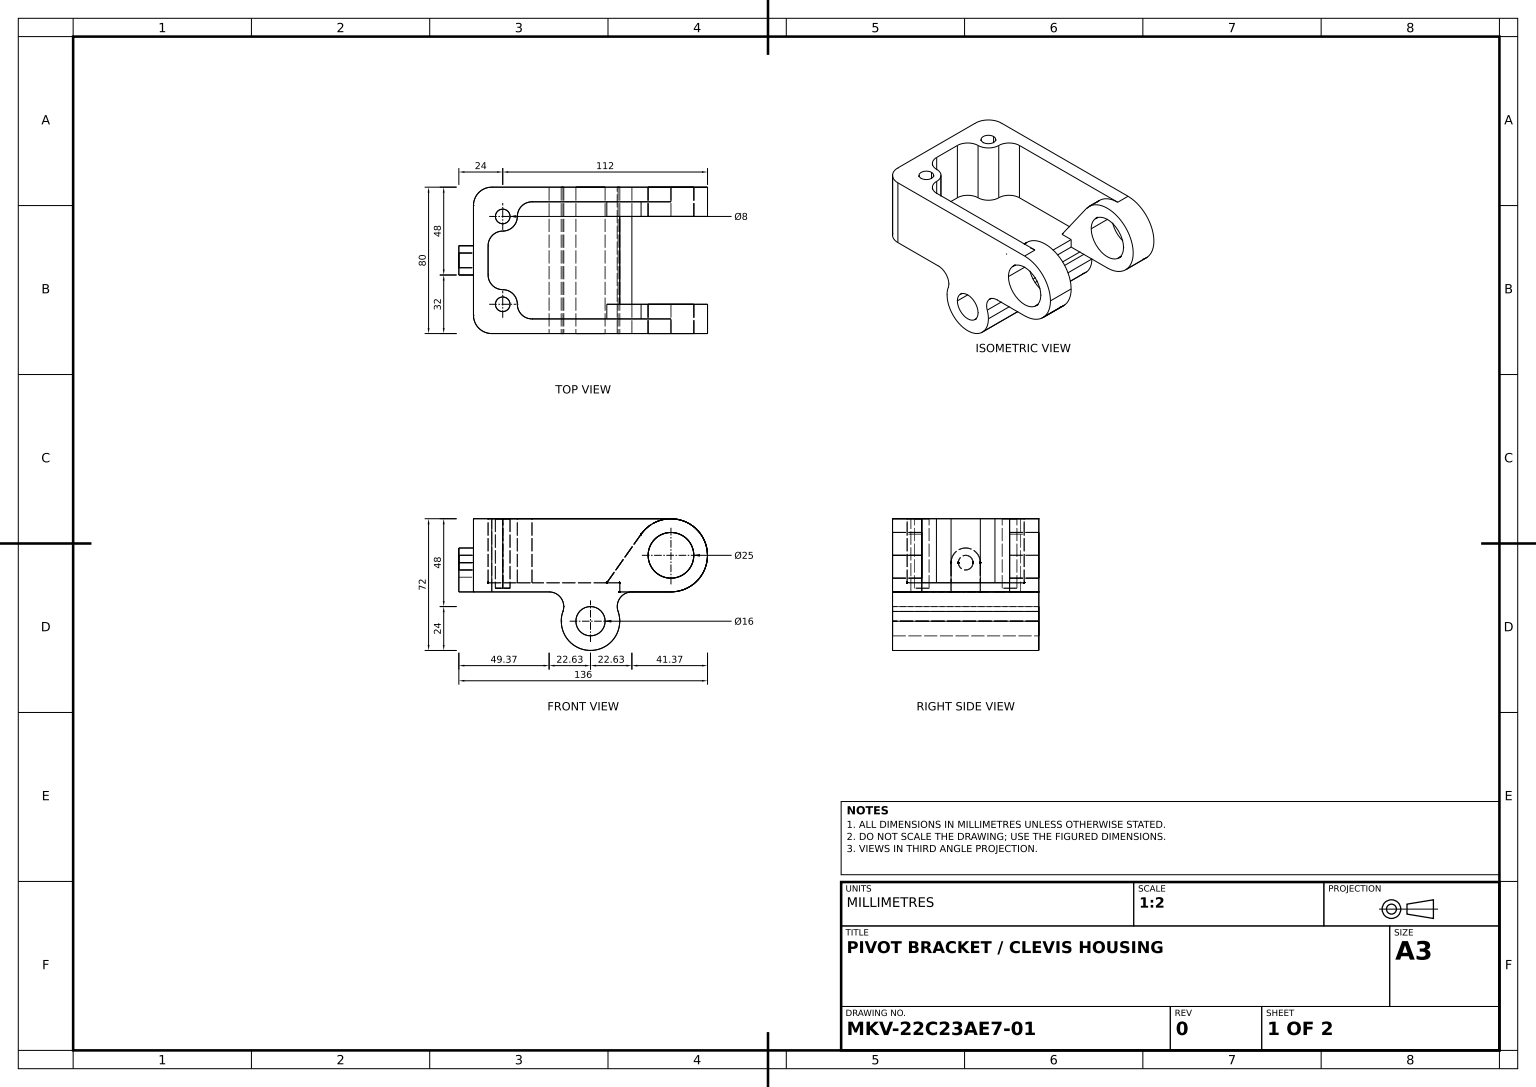
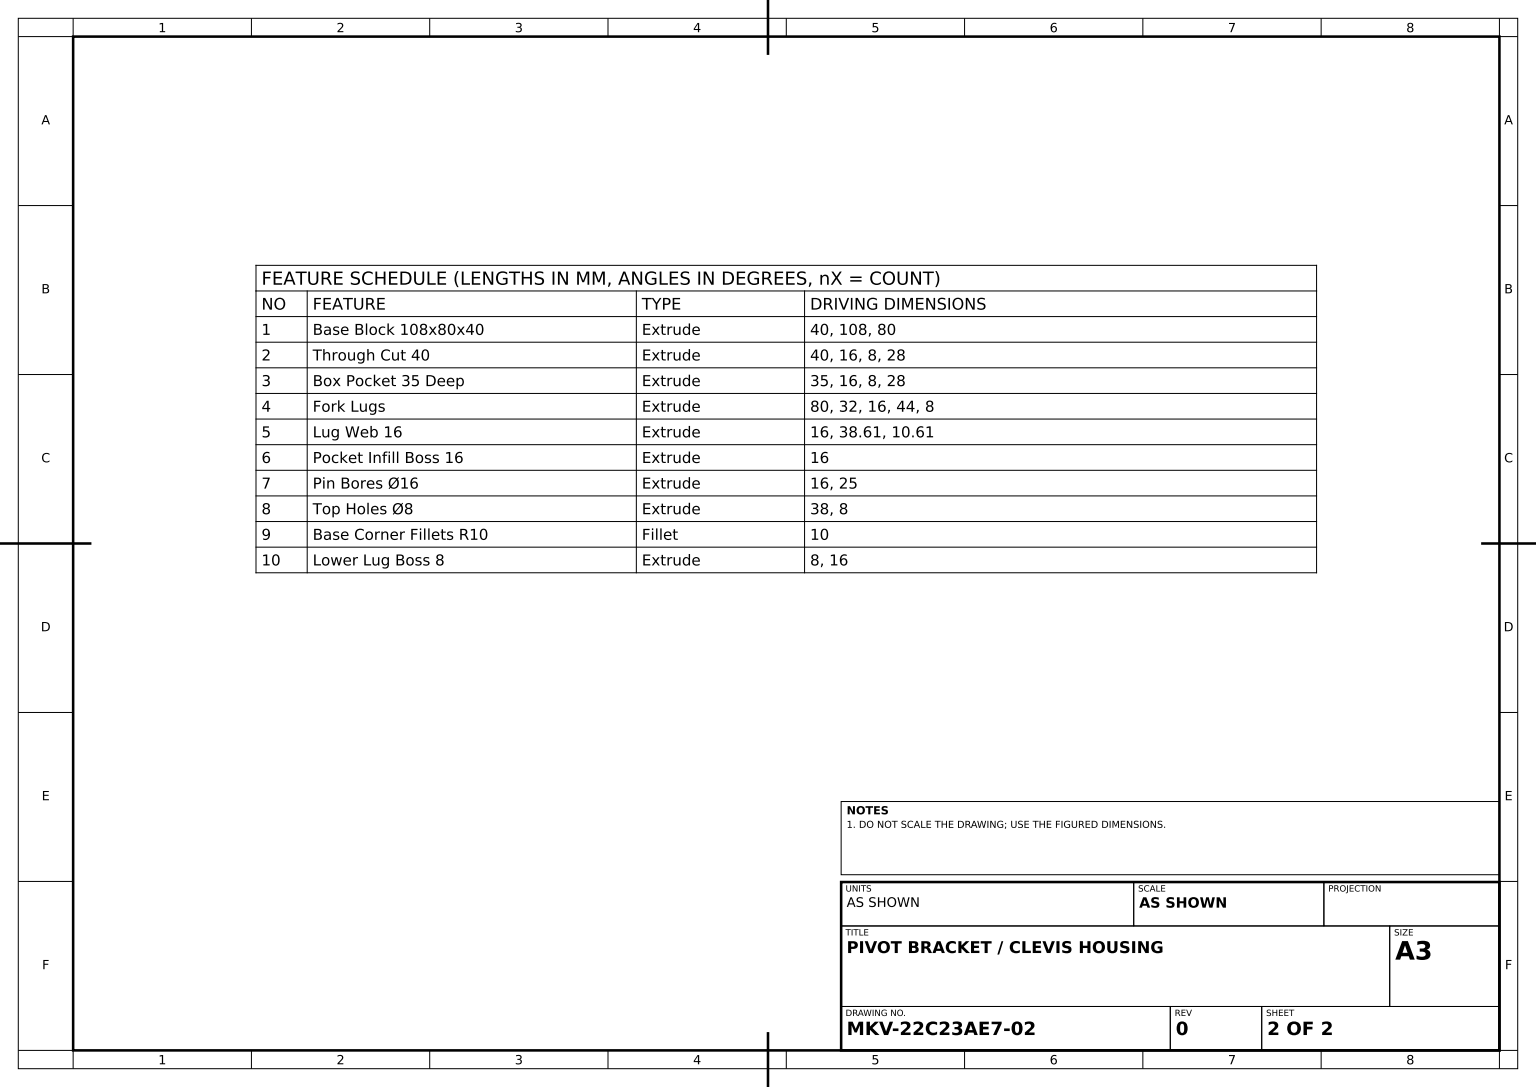
from build123d import *

# Parameters (mm, degrees)
BASE_BLOCK_SKETCH_W         = 108
BASE_BLOCK_SKETCH_H         = 80
BASE_BLOCK_108X80X40_DEPTH  = 40
BOX_POCKET_SKETCH_W         = 28
BOX_POCKET_SKETCH_H         = 32
THROUGH_CUT_40_DEPTH        = 40
BOX_POCKET_35_DEEP_DEPTH    = 35
FORK_LUGS_DEPTH             = 80
LUG_WEB_16_DEPTH            = 16
POCKET_START                = -16
POCKET_INFILL_BOSS_16_DEPTH = 16
PIN_BORE_SKETCH_R           = 12.5
PIN_BORE_SKETCH_R_2         = 8
PIN_BORES_16_DEPTH          = 117.086174887
TOP_HOLES_SKETCH_R          = 4
TOP_HOLES_8_DEPTH           = 38
BASE_CORNER_FILLETS_R10_R   = 10
LOWER_LUG_SKETCH_R          = 4
LOWER_LUG_BOSS_8_DEPTH      = 8


with BuildPart() as part:
    # Base Block Sketch → Base Block 108x80x40 (new body)
    with BuildSketch(Plane(origin=(0, 0, 0), x_dir=(1, 0, 0), z_dir=(0, 1, 0))):
        Rectangle(BASE_BLOCK_SKETCH_W, BASE_BLOCK_SKETCH_H)
    extrude(amount=BASE_BLOCK_108X80X40_DEPTH)

    # Box Pocket Sketch → Through Cut 40 (cut)
    with BuildSketch(Plane(origin=(0, 40, 0), x_dir=(1, 0, 0), z_dir=(0, 1, 0))):
        with Locations((40, -16)):
            Rectangle(BOX_POCKET_SKETCH_W, BOX_POCKET_SKETCH_H)
        with Locations((40, 16)):
            Rectangle(BOX_POCKET_SKETCH_W, BOX_POCKET_SKETCH_H)
    extrude(amount=-THROUGH_CUT_40_DEPTH, mode=Mode.SUBTRACT)

    # Sketch3_3 → Box Pocket 35 Deep (cut)
    with BuildSketch(Plane(origin=(0, 40, 0), x_dir=(1, 0, 0), z_dir=(0, 1, 0))):
        with BuildLine():
            Line((-22, -32), (26, -32))
            Line((26, -32), (26, 32))
            Line((26, 32), (-22, 32))
            ThreePointArc((-22, 32), (-27.656854249, 29.656854249), (-30, 24))
            ThreePointArc((-30, 24), (-32.343145751, 18.343145751), (-38, 16))
            ThreePointArc((-38, 16), (-43.656854249, 13.656854249), (-46, 8))
            Line((-46, 8), (-46, -8))
            ThreePointArc((-46, -8), (-43.656854249, -13.656854249), (-38, -16))
            ThreePointArc((-38, -16), (-32.343145751, -18.343145751), (-30, -24))
            ThreePointArc((-30, -24), (-27.656854249, -29.656854249), (-22, -32))
        make_face()
    extrude(amount=-BOX_POCKET_35_DEEP_DEPTH, mode=Mode.SUBTRACT)

    # Fork Lug Sketch → Fork Lugs (add)
    with BuildSketch(Plane.XY.offset(40)):
        with BuildLine():
            Line((-12.627416998, 0), (32.627416998, 0))
            ThreePointArc((32.627416998, 0), (26.095444351, -3.381197846), (25.084944665, -10.666666667))
            ThreePointArc((25.084944665, -10.666666667), (10, -32), (-5.084944665, -10.666666667))
            ThreePointArc((-5.084944665, -10.666666667), (-6.095444351, -3.381197846), (-12.627416998, 0))
        make_face()
    extrude(amount=-FORK_LUGS_DEPTH)

    # Lug Web Sketch → Lug Web 16 (add)
    with BuildSketch(Plane.XY.offset(40)):
        with BuildLine():
            Line((37.663470885, 31.537669456), (15.39, 0))
            Line((15.39, 0), (26, 0))
            Line((26, 0), (26.095444351, -3.381197846))
            ThreePointArc((26.095444351, -3.381197846), (28.949810251, -0.895409328), (32.627416998, 0))
            Line((32.627416998, 0), (54, 0))
            ThreePointArc((54, 0), (71.758848346, 29.199092642), (37.663470885, 31.537669456))
        make_face()
    extrude(amount=-LUG_WEB_16_DEPTH)

    # Pocket Infill Sketch → Pocket Infill Boss 16 (add)
    with BuildSketch(Plane(origin=(0, 0, -40), x_dir=(-1, 0, 0), z_dir=(0, 0, -1)).offset(POCKET_START)):
        with BuildLine():
            Line((-32.627416998, 0), (-54, 0))
            ThreePointArc((-54, 0), (-74, 20), (-54, 40))
            ThreePointArc((-54, 40), (-44.800907358, 37.758848346), (-37.663470885, 31.537669456))
            Line((-37.663470885, 31.537669456), (-18.921248705, 5))
            Line((-18.921248705, 5), (-26, 5))
            Line((-26, 5), (-26, -3.519225074))
            ThreePointArc((-26, -3.519225074), (-28.87549745, -0.934371953), (-32.627416998, 0))
        make_face()
    extrude(amount=POCKET_INFILL_BOSS_16_DEPTH)

    # Pin Bore Sketch → Pin Bores _16 (cut, through all)
    with BuildSketch(Plane.XY.offset(40)):
        with Locations((54, 20)):
            Circle(PIN_BORE_SKETCH_R)
        with Locations((10, -16)):
            Circle(PIN_BORE_SKETCH_R_2)
    extrude(amount=-PIN_BORES_16_DEPTH, mode=Mode.SUBTRACT)

    # Top Holes Sketch → Top Holes _8 (cut)
    with BuildSketch(Plane(origin=(0, 40, 0), x_dir=(1, 0, 0), z_dir=(0, 1, 0))):
        with Locations(Location((-38, 24, 0), (0, 0, 270))):
            Circle(TOP_HOLES_SKETCH_R)
        with Locations(Location((-38, -24, 0), (0, 0, 270))):
            Circle(TOP_HOLES_SKETCH_R)
    extrude(amount=-TOP_HOLES_8_DEPTH, mode=Mode.SUBTRACT)

    # Base Corner Fillets R10
    base_corner_fillets_r10_edges = [part.edges().sort_by_distance(p)[0] for p in [
        (-54, 20, 40),
        (-54, 20, -40),
    ]]
    fillet(base_corner_fillets_r10_edges, radius=BASE_CORNER_FILLETS_R10_R)

    # Lower Lug Sketch → Lower Lug Boss 8 (add)
    with BuildSketch(Plane.ZY.offset(54)):
        with BuildLine():
            Line((-8, 16), (-8, 0))
            Line((-8, 0), (8, 0))
            Line((8, 0), (8, 16))
            ThreePointArc((8, 16), (0, 24), (-8, 16))
        make_face()
        with Locations((0, 16)):
            Circle(LOWER_LUG_SKETCH_R, mode=Mode.SUBTRACT)
    extrude(amount=LOWER_LUG_BOSS_8_DEPTH)


solid = part.part
